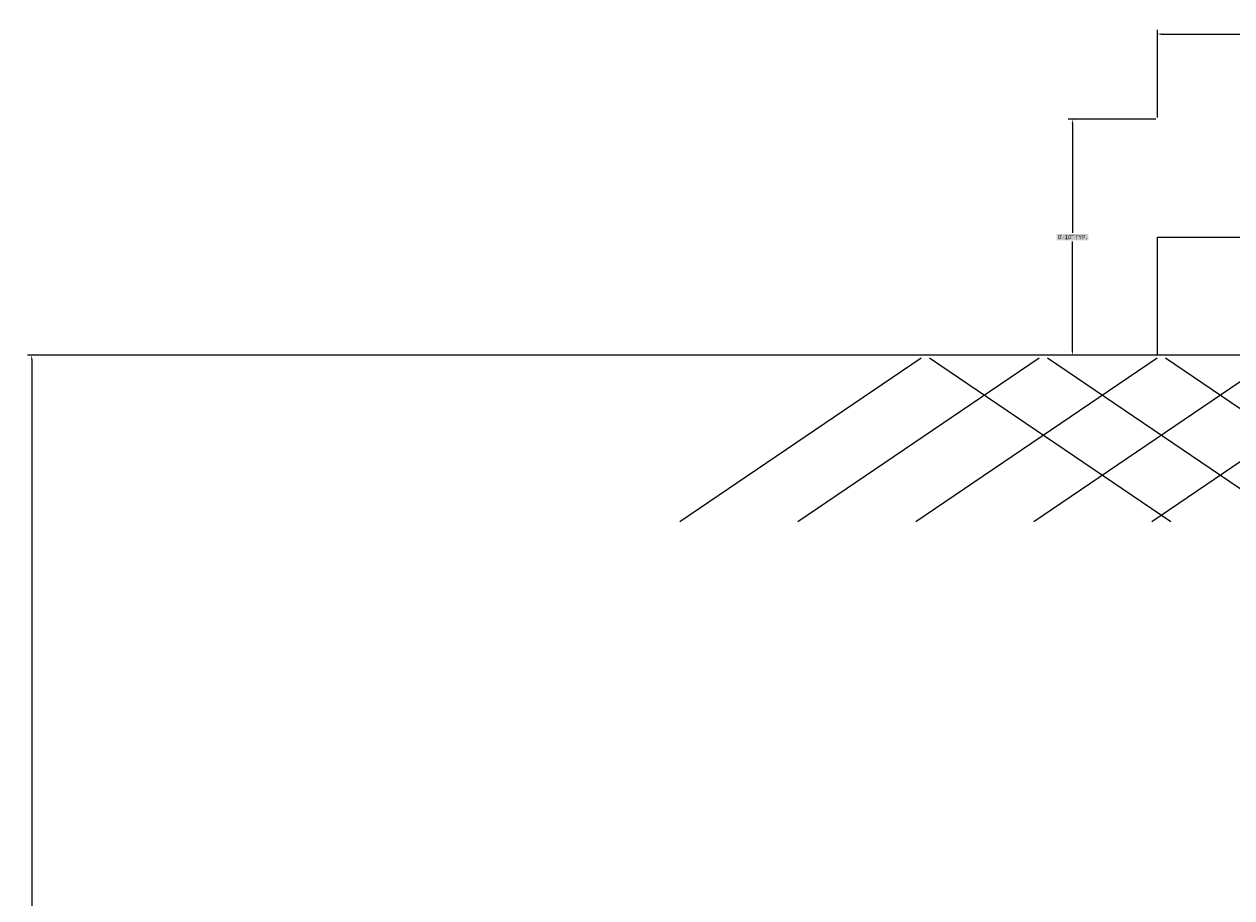
# Model space of a CAD drawing. Units: inches. Extents: x -128 to 854, y -395 to 398.
# Tile 2 of 61: x -128 to -77, y -321 to -284. Entities that reach past the tile are written whole.
import ezdxf

# ---------------------------------------------------------------- set-up
doc = ezdxf.new("R2010")
doc.units = ezdxf.units.IN
doc.header["$MEASUREMENT"] = 0
for name, color, linetype, lineweight in [('A-ANNO-DIMS', 2, 'Continuous', 18), ('A-FLOR-STRS', 7, 'Continuous', 25), ('C-GRAD', 7, 'Continuous', 25), ('C-GRAD-PATT', 8, 'Continuous', 13)]:
    doc.layers.add(name, color=color, linetype=linetype, lineweight=lineweight)
doc.styles.get("Standard").update_dxf_attribs({"font": 'arial.ttf'})
doc.dimstyles.get("Standard").update_dxf_attribs({"dimtxt": 0.18, "dimasz": 0.18, "dimexe": 0.18, "dimexo": 0.0625, "dimgap": 0.09, "dimtad": 0, "dimtih": 1, "dimtoh": 1, "dimdec": 1, "dimzin": 0, "dimdsep": 46, "dimlunit": 4, "dimtxsty": 'Standard', "dimcen": 0.09, "dimclrd": 1, "dimclre": 2, "dimclrt": 6, "dimadec": 0, "dimazin": 0, "dimtfac": 1, "dimtdec": 1, "dimtofl": 0, "dimtmove": 0, "dimatfit": 3, "dimfxl": 1, "dimtfill": 2, "dimtfillclr": 3, "dimtolj": 1, "dimtzin": 0, "dimarcsym": 0})

# ---------------------------------------------------------------- blocks, each defined once
blk = doc.blocks.new('ENTRY-STEPS-SECTION')
for p, q in [((12, 5), (12, 10)), ((12, 10), (24, 10)), ((0, 0), (0, 5)), ((0, 5), (12, 5)), ((24, 0), (0, 0))]:
    blk.add_line(p, q)
blk = doc.blocks.new('*D89')
at = {"layer": 'A-ANNO-DIMS', "color": 2, "lineweight": -2, "transparency": 16777216}
for p, q in [((-80.161, -287.957), (-80.161, -284.239)), ((-56.161, -287.957), (-56.161, -284.239))]:
    blk.add_line(p, q, dxfattribs=at)
at = {"layer": 'A-ANNO-DIMS', "color": 1, "lineweight": -2, "transparency": 16777216}
for p, q in [((-79.981, -284.419), (-69.246, -284.419)), ((-56.341, -284.419), (-67.076, -284.419))]:
    blk.add_line(p, q, dxfattribs=at)
at = {"layer": 'A-ANNO-DIMS', "color": 1, "transparency": 16777216}
for points in [[(-79.981, -284.389), (-79.981, -284.449), (-80.161, -284.419)], [(-56.341, -284.389), (-56.341, -284.449), (-56.161, -284.419)]]:
    blk.add_solid(points, dxfattribs=at)
at = {"layer": 'Defpoints', "color": 0, "transparency": 16777216}
for p in [(-56.161, -284.419), (-80.161, -288.019), (-56.161, -288.019)]:
    blk.add_point(p, dxfattribs=at)
at = {"layer": 'A-ANNO-DIMS', "color": 6, "transparency": 16777216, "insert": (-68.161, -284.419), "char_height": 0.18, "attachment_point": 5, "bg_fill": 1, "box_fill_scale": 1.25, "bg_fill_color": 3, "bg_fill_transparency": 0}
blk.add_mtext('\\A1;STEPS 2\'-0" TYP.', dxfattribs=at)
blk = doc.blocks.new('*D90')
at = {"layer": 'A-ANNO-DIMS', "color": 2, "lineweight": -2, "transparency": 16777216}
for p, q in [((-80.223, -288.019), (-83.941, -288.019)), ((-80.223, -298.019), (-83.941, -298.019))]:
    blk.add_line(p, q, dxfattribs=at)
at = {"layer": 'A-ANNO-DIMS', "color": 1, "lineweight": -2, "transparency": 16777216}
for p, q in [((-83.761, -288.199), (-83.761, -292.837)), ((-83.761, -297.839), (-83.761, -293.201))]:
    blk.add_line(p, q, dxfattribs=at)
at = {"layer": 'A-ANNO-DIMS', "color": 1, "transparency": 16777216}
for points in [[(-83.791, -288.199), (-83.731, -288.199), (-83.761, -288.019)], [(-83.791, -297.839), (-83.731, -297.839), (-83.761, -298.019)]]:
    blk.add_solid(points, dxfattribs=at)
at = {"layer": 'Defpoints', "color": 0, "transparency": 16777216}
for p in [(-83.761, -288.019), (-80.161, -288.019), (-80.161, -298.019)]:
    blk.add_point(p, dxfattribs=at)
at = {"layer": 'A-ANNO-DIMS', "color": 6, "transparency": 16777216, "insert": (-83.761, -293.019), "char_height": 0.18, "attachment_point": 5, "bg_fill": 1, "box_fill_scale": 1.25, "bg_fill_color": 3, "bg_fill_transparency": 0}
blk.add_mtext('\\A1;0\'-10" TYP.', dxfattribs=at)
blk = doc.blocks.new('*D121')
at = {"layer": 'A-ANNO-DIMS', "color": 2, "lineweight": -2, "transparency": 16777216}
for p, q in [((-56.223, -298.019), (-128.041, -298.019)), ((-76.223, -358.019), (-128.041, -358.019))]:
    blk.add_line(p, q, dxfattribs=at)
at = {"layer": 'A-ANNO-DIMS', "color": 1, "lineweight": -2, "transparency": 16777216}
for p, q in [((-127.861, -298.199), (-127.861, -327.837)), ((-127.861, -357.839), (-127.861, -328.201))]:
    blk.add_line(p, q, dxfattribs=at)
at = {"layer": 'A-ANNO-DIMS', "color": 1, "transparency": 16777216}
for points in [[(-127.891, -298.199), (-127.831, -298.199), (-127.861, -298.019)], [(-127.891, -357.839), (-127.831, -357.839), (-127.861, -358.019)]]:
    blk.add_solid(points, dxfattribs=at)
at = {"layer": 'Defpoints', "color": 0, "transparency": 16777216}
for p in [(-56.161, -298.019), (-127.861, -358.019), (-76.161, -358.019)]:
    blk.add_point(p, dxfattribs=at)
at = {"layer": 'A-ANNO-DIMS', "color": 6, "transparency": 16777216, "insert": (-127.861, -328.019), "char_height": 0.18, "attachment_point": 5, "bg_fill": 1, "box_fill_scale": 1.25, "bg_fill_color": 3, "bg_fill_transparency": 0}
blk.add_mtext('\\A1;5\'-0"', dxfattribs=at)

msp = doc.modelspace()

# ---------------------------------------------------------------- hatches: boundary and pattern name
at = {"layer": 'C-GRAD-PATT'}
h = msp.add_hatch(dxfattribs=at)
h.set_pattern_fill('ANSI31', color=256, scale=22.43157, angle=349.1104, style=0)
h.paths.add_polyline_path([(-94.192, -298.137), (-69.212, -298.137), (-79.439, -305.063), (-104.419, -305.063)])
h = msp.add_hatch(dxfattribs=at)
h.set_pattern_fill('ANSI31', color=256, scale=22.43157, angle=100.8896, style=0)
h.paths.add_polyline_path([(-94.192, -298.137), (-69.212, -298.137), (-58.986, -305.063), (-83.966, -305.063)])

# ---------------------------------------------------------------- linework, layer by layer
at = {"layer": 'C-GRAD'}
msp.add_line((-56.161, -298.019), (-104.161, -298.019), dxfattribs=at)

# ---------------------------------------------------------------- block references
at = {"layer": 'A-FLOR-STRS'}
msp.add_blockref('ENTRY-STEPS-SECTION', (-80.161, -298.019), dxfattribs=at)

# ---------------------------------------------------------------- dimensions: what is measured, and where the dimension line sits
at = {"layer": 'A-ANNO-DIMS'}
dim = msp.add_linear_dim(base=(-56.161, -284.419), p1=(-80.161, -288.019), p2=(-56.161, -288.019), text='STEPS <> TYP.', dimstyle='Standard', override={"dimdec": 1, "dimlfac": 1, "dimrnd": 0, "dimzin": 1, "dimdsep": 46, "dimlunit": 4, "dimfrac": 2}, dxfattribs=at)
dim.commit()
dim.dimension.update_dxf_attribs({"geometry": '*D89', "text_midpoint": (-68.161, -284.419)})
dim = msp.add_linear_dim(base=(-83.761, -288.019), p1=(-80.161, -298.019), p2=(-80.161, -288.019), angle=90, text='<> TYP.', dimstyle='Standard', override={"dimdec": 1, "dimlfac": 1, "dimrnd": 0, "dimzin": 1, "dimdsep": 46, "dimlunit": 4, "dimfrac": 2}, dxfattribs=at)
dim.commit()
dim.dimension.update_dxf_attribs({"geometry": '*D90', "text_midpoint": (-83.761, -293.019)})
dim = msp.add_linear_dim(base=(-127.861, -358.019), p1=(-56.161, -298.019), p2=(-76.161, -358.019), angle=90, dimstyle='Standard', override={"dimdec": 1, "dimlfac": 1, "dimrnd": 0, "dimzin": 1, "dimdsep": 46, "dimlunit": 4, "dimfrac": 2}, dxfattribs=at)
dim.commit()
dim.dimension.update_dxf_attribs({"geometry": '*D121', "text_midpoint": (-127.861, -328.019)})

doc.saveas('drawing.dxf')
